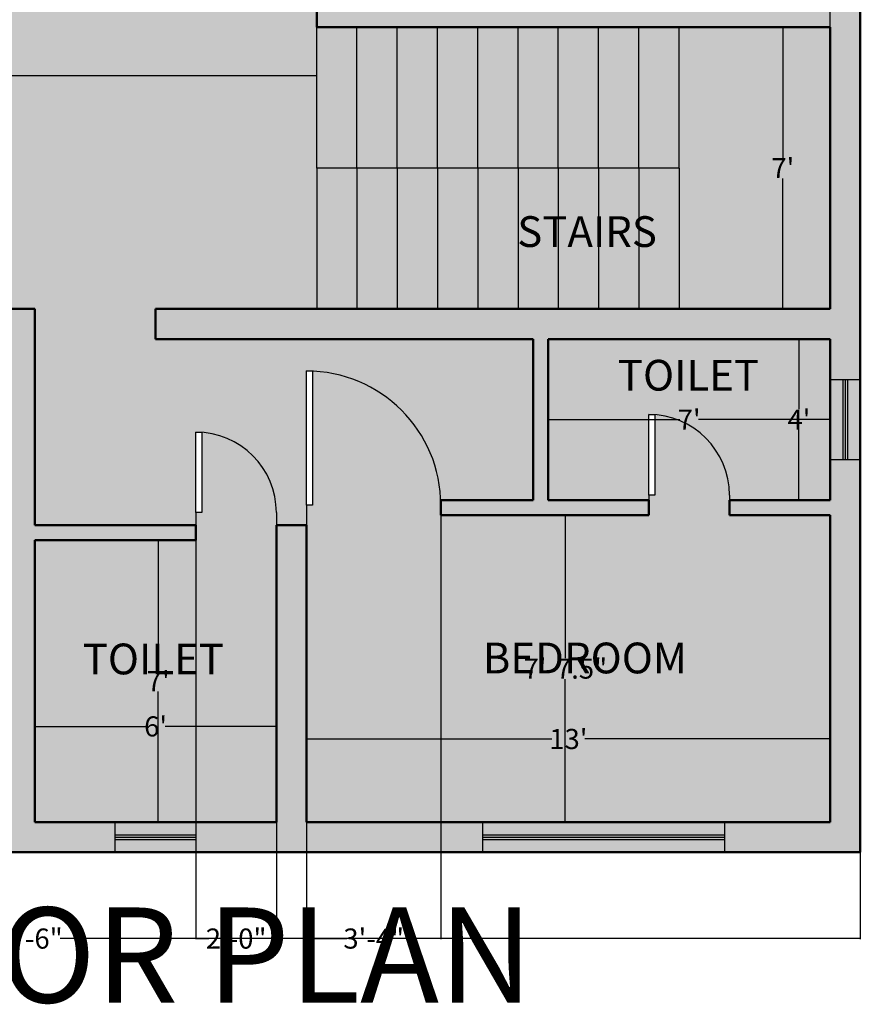
# Model space of a CAD drawing. Units: inches. Extents: x 1379 to 6665, y -118 to 1026.
# Tile 28 of 29: x 6415 to 6665, y 26 to 320. Entities that reach past the tile are written whole.
import ezdxf

# ---------------------------------------------------------------- set-up
doc = ezdxf.new("R2010")
doc.units = ezdxf.units.IN
doc.header["$MEASUREMENT"] = 0
for name, color, linetype, lineweight in [('A-ANNO-DIMS', 2, 'Continuous', 18), ('A-ANNO-TEXT', 7, 'Continuous', 35), ('A-AREA-IDEN', 7, 'Continuous', 25), ('A-DOOR', 1, 'Continuous', 25), ('A-FLOR-PATT', 252, 'Continuous', 13), ('A-FLOR-STRS', 131, 'Continuous', 25), ('A-GLAZ', 2, 'Continuous', 25), ('A-WALL', 7, 'Continuous', 50), ('A-WALL-PATT', 8, 'Continuous', 13)]:
    doc.layers.add(name, color=color, linetype=linetype, lineweight=lineweight)
doc.styles.get("Standard").update_dxf_attribs({"font": 'arial.ttf'})
doc.dimstyles.get("Standard").update_dxf_attribs({"dimtxt": 6, "dimasz": 0.18, "dimexe": 0.18, "dimexo": 0.0625, "dimgap": 0.09, "dimtad": 0, "dimtih": 1, "dimtoh": 1, "dimdec": 1, "dimzin": 0, "dimdsep": 46, "dimlunit": 3, "dimtxsty": 'Standard', "dimcen": 0.09, "dimclrt": 250, "dimadec": 0, "dimazin": 0, "dimtfac": 1, "dimtdec": 1, "dimtofl": 0, "dimtmove": 0, "dimatfit": 3, "dimfxl": 1, "dimtolj": 1, "dimtzin": 0, "dimarcsym": 0})

# ---------------------------------------------------------------- blocks, each defined once
blk = doc.blocks.new('*D79')
at = {"layer": 'A-ANNO-DIMS', "color": 0, "lineweight": -2, "transparency": 16777216}
for p, q in [((6640.02, 317.64), (6642.5, 317.64)), ((6642.32, 317.46), (6642.32, 278.73)), ((6642.32, 233.82), (6642.32, 272.55)), ((6640.02, 233.64), (6642.5, 233.64))]:
    blk.add_line(p, q, dxfattribs=at)
at = {"layer": 'A-ANNO-DIMS', "color": 0, "transparency": 16777216}
for points in [[(6642.29, 317.46), (6642.35, 317.46), (6642.32, 317.64)], [(6642.29, 233.82), (6642.35, 233.82), (6642.32, 233.64)]]:
    blk.add_solid(points, dxfattribs=at)
at = {"layer": 'Defpoints', "color": 0, "transparency": 16777216}
for p in [(6639.95, 317.64), (6639.95, 233.64), (6642.32, 233.64)]:
    blk.add_point(p, dxfattribs=at)
at = {"layer": 'A-ANNO-DIMS', "color": 0, "transparency": 16777216, "insert": (6642.32, 275.64), "char_height": 6, "attachment_point": 5}
blk.add_mtext("\\A1;7'", dxfattribs=at)
blk = doc.blocks.new('*U2')
for p, q in [((0, 0), (0, -6)), ((24, 0), (24, -6))]:
    blk.add_line(p, q)
blk.add_lwpolyline([(0, 0), (0, 24), (1.75, 24), (1.75, 0)], close=True)
blk.add_arc((0, 0), 24, 0, 90)
blk = doc.blocks.new('*U25')
for p, q in [((0, 0), (0, -6)), ((40, 0), (40, -6))]:
    blk.add_line(p, q)
blk.add_lwpolyline([(0, 0), (0, 40), (1.75, 40), (1.75, 0)], close=True)
blk.add_arc((0, 0), 40, 0, 90)
blk = doc.blocks.new('*D80')
at = {"layer": 'A-ANNO-DIMS', "color": 0, "lineweight": -2, "transparency": 16777216}
for p, q in [((6176.4, 282.22), (6176.4, 303.33)), ((6176.58, 303.15), (6325.96, 303.15)), ((6503.22, 303.15), (6353.84, 303.15)), ((6503.4, 282.22), (6503.4, 303.33))]:
    blk.add_line(p, q, dxfattribs=at)
at = {"layer": 'A-ANNO-DIMS', "color": 0, "transparency": 16777216}
for points in [[(6176.58, 303.18), (6176.58, 303.12), (6176.4, 303.15)], [(6503.22, 303.18), (6503.22, 303.12), (6503.4, 303.15)]]:
    blk.add_solid(points, dxfattribs=at)
at = {"layer": 'Defpoints', "color": 0, "transparency": 16777216}
for p in [(6503.4, 303.15), (6176.4, 282.16), (6503.4, 282.16)]:
    blk.add_point(p, dxfattribs=at)
at = {"layer": 'A-ANNO-DIMS', "color": 0, "transparency": 16777216, "insert": (6339.9, 303.15), "char_height": 6, "attachment_point": 5}
blk.add_mtext('\\A1;27\'-3.0"', dxfattribs=at)
blk = doc.blocks.new('*D70')
at = {"layer": 'A-ANNO-DIMS', "color": 0, "lineweight": -2, "transparency": 16777216}
for p, q in [((6453.93, 164.64), (6456.37, 164.64)), ((6456.19, 164.46), (6456.19, 125.73)), ((6456.19, 80.82), (6456.19, 119.55)), ((6453.93, 80.64), (6456.37, 80.64))]:
    blk.add_line(p, q, dxfattribs=at)
at = {"layer": 'A-ANNO-DIMS', "color": 0, "transparency": 16777216}
for points in [[(6456.16, 164.46), (6456.22, 164.46), (6456.19, 164.64)], [(6456.16, 80.82), (6456.22, 80.82), (6456.19, 80.64)]]:
    blk.add_solid(points, dxfattribs=at)
at = {"layer": 'Defpoints', "color": 0, "transparency": 16777216}
for p in [(6453.87, 164.64), (6453.87, 80.64), (6456.19, 80.64)]:
    blk.add_point(p, dxfattribs=at)
at = {"layer": 'A-ANNO-DIMS', "color": 0, "transparency": 16777216, "insert": (6456.19, 122.64), "char_height": 6, "attachment_point": 5}
blk.add_mtext("\\A1;7'", dxfattribs=at)
blk = doc.blocks.new('*D71')
at = {"layer": 'A-ANNO-DIMS', "color": 0, "lineweight": -2, "transparency": 16777216}
for p, q in [((6419.4, 114.02), (6419.4, 108.98)), ((6419.58, 109.16), (6452.54, 109.16)), ((6491.22, 109.16), (6458.27, 109.16)), ((6491.4, 109.22), (6491.4, 109.34))]:
    blk.add_line(p, q, dxfattribs=at)
at = {"layer": 'A-ANNO-DIMS', "color": 0, "transparency": 16777216}
for points in [[(6419.58, 109.19), (6419.58, 109.13), (6419.4, 109.16)], [(6491.22, 109.19), (6491.22, 109.13), (6491.4, 109.16)]]:
    blk.add_solid(points, dxfattribs=at)
at = {"layer": 'Defpoints', "color": 0, "transparency": 16777216}
for p in [(6419.4, 114.09), (6491.4, 109.16), (6491.4, 109.16)]:
    blk.add_point(p, dxfattribs=at)
at = {"layer": 'A-ANNO-DIMS', "color": 0, "transparency": 16777216, "insert": (6455.4, 109.16), "char_height": 6, "attachment_point": 5}
blk.add_mtext("\\A1;6'", dxfattribs=at)
blk = doc.blocks.new('*D72')
at = {"layer": 'A-ANNO-DIMS', "color": 0, "lineweight": -2, "transparency": 16777216}
for p, q in [((6578.31, 172.14), (6577.32, 172.14)), ((6577.5, 171.96), (6577.5, 129.53)), ((6577.5, 80.82), (6577.5, 123.25)), ((6578.31, 80.64), (6577.32, 80.64))]:
    blk.add_line(p, q, dxfattribs=at)
at = {"layer": 'A-ANNO-DIMS', "color": 0, "transparency": 16777216}
for points in [[(6577.47, 171.96), (6577.53, 171.96), (6577.5, 172.14)], [(6577.47, 80.82), (6577.53, 80.82), (6577.5, 80.64)]]:
    blk.add_solid(points, dxfattribs=at)
at = {"layer": 'Defpoints', "color": 0, "transparency": 16777216}
for p in [(6578.37, 172.14), (6577.5, 80.64), (6578.37, 80.64)]:
    blk.add_point(p, dxfattribs=at)
at = {"layer": 'A-ANNO-DIMS', "color": 0, "transparency": 16777216, "insert": (6577.5, 126.39), "char_height": 6, "attachment_point": 5}
blk.add_mtext('\\A1;7\'-7.5"', dxfattribs=at)
blk = doc.blocks.new('*D73')
at = {"layer": 'A-ANNO-DIMS', "color": 0, "lineweight": -2, "transparency": 16777216}
for p, q in [((6500.4, 124.83), (6500.4, 105.22)), ((6656.4, 124.83), (6656.4, 105.22)), ((6500.58, 105.4), (6573.5, 105.4)), ((6656.22, 105.4), (6583.3, 105.4))]:
    blk.add_line(p, q, dxfattribs=at)
at = {"layer": 'A-ANNO-DIMS', "color": 0, "transparency": 16777216}
for points in [[(6500.58, 105.43), (6500.58, 105.37), (6500.4, 105.4)], [(6656.22, 105.43), (6656.22, 105.37), (6656.4, 105.4)]]:
    blk.add_solid(points, dxfattribs=at)
at = {"layer": 'Defpoints', "color": 0, "transparency": 16777216}
for p in [(6500.4, 124.89), (6656.4, 124.89), (6656.4, 105.4)]:
    blk.add_point(p, dxfattribs=at)
at = {"layer": 'A-ANNO-DIMS', "color": 0, "transparency": 16777216, "insert": (6578.4, 105.4), "char_height": 6, "attachment_point": 5}
blk.add_mtext("\\A1;13'", dxfattribs=at)
blk = doc.blocks.new('*D74')
at = {"layer": 'A-ANNO-DIMS', "color": 0, "lineweight": -2, "transparency": 16777216}
for p, q in [((6647.16, 224.64), (6646.93, 224.64)), ((6647.11, 224.46), (6647.11, 203.73)), ((6647.11, 176.82), (6647.11, 197.55)), ((6647.16, 176.64), (6646.93, 176.64))]:
    blk.add_line(p, q, dxfattribs=at)
at = {"layer": 'A-ANNO-DIMS', "color": 0, "transparency": 16777216}
for points in [[(6647.08, 224.46), (6647.14, 224.46), (6647.11, 224.64)], [(6647.08, 176.82), (6647.14, 176.82), (6647.11, 176.64)]]:
    blk.add_solid(points, dxfattribs=at)
at = {"layer": 'Defpoints', "color": 0, "transparency": 16777216}
for p in [(6647.23, 224.64), (6647.11, 176.64), (6647.23, 176.64)]:
    blk.add_point(p, dxfattribs=at)
at = {"layer": 'A-ANNO-DIMS', "color": 0, "transparency": 16777216, "insert": (6647.11, 200.64), "char_height": 6, "attachment_point": 5}
blk.add_mtext("\\A1;4'", dxfattribs=at)
blk = doc.blocks.new('*D75')
at = {"layer": 'A-ANNO-DIMS', "color": 0, "lineweight": -2, "transparency": 16777216}
for p, q in [((6572.4, 194.48), (6572.4, 200.82)), ((6572.58, 200.64), (6611.58, 200.64)), ((6656.22, 200.64), (6617.23, 200.64)), ((6656.4, 191.52), (6656.4, 200.82))]:
    blk.add_line(p, q, dxfattribs=at)
at = {"layer": 'A-ANNO-DIMS', "color": 0, "transparency": 16777216}
for points in [[(6572.58, 200.67), (6572.58, 200.61), (6572.4, 200.64)], [(6656.22, 200.67), (6656.22, 200.61), (6656.4, 200.64)]]:
    blk.add_solid(points, dxfattribs=at)
at = {"layer": 'Defpoints', "color": 0, "transparency": 16777216}
for p in [(6656.4, 200.64), (6572.4, 194.41), (6656.4, 191.46)]:
    blk.add_point(p, dxfattribs=at)
at = {"layer": 'A-ANNO-DIMS', "color": 0, "transparency": 16777216, "insert": (6614.4, 200.64), "char_height": 6, "attachment_point": 5}
blk.add_mtext("\\A1;7'", dxfattribs=at)
blk = doc.blocks.new('WIN-1800')
for p, q in [((0, 0.73), (72, 0.73)), ((0, 0), (72, 0))]:
    blk.add_line(p, q)
blk = doc.blocks.new('WIN-600')
for p, q in [((0, 24), (0, 0)), ((0.73, 24), (0.73, 0))]:
    blk.add_line(p, q)
blk = doc.blocks.new('*D136')
at = {"layer": 'A-ANNO-DIMS', "color": 0, "lineweight": -2, "transparency": 16777216}
for p, q in [((6167.4, 71.58), (6167.4, 45.71)), ((6665.4, 71.58), (6665.4, 45.71)), ((6167.58, 45.89), (6405.89, 45.89)), ((6665.22, 45.89), (6426.92, 45.89))]:
    blk.add_line(p, q, dxfattribs=at)
at = {"layer": 'A-ANNO-DIMS', "color": 0, "transparency": 16777216}
for points in [[(6167.58, 45.92), (6167.58, 45.86), (6167.4, 45.89)], [(6665.22, 45.92), (6665.22, 45.86), (6665.4, 45.89)]]:
    blk.add_solid(points, dxfattribs=at)
at = {"layer": 'Defpoints', "color": 0, "transparency": 16777216}
for p in [(6167.4, 71.64), (6665.4, 71.64), (6665.4, 45.89)]:
    blk.add_point(p, dxfattribs=at)
at = {"layer": 'A-ANNO-DIMS', "color": 250, "transparency": 16777216, "insert": (6416.4, 45.89), "char_height": 6, "attachment_point": 5}
blk.add_mtext('\\A1;41\'-6"', dxfattribs=at)
blk = doc.blocks.new('*D142')
at = {"layer": 'A-ANNO-DIMS', "color": 0, "lineweight": -2, "transparency": 16777216}
for p, q in [((6503.4, 317.7), (6503.4, 529.57)), ((6503.58, 529.39), (6569.79, 529.39)), ((6656.22, 529.39), (6590.02, 529.39)), ((6656.4, 317.7), (6656.4, 529.57))]:
    blk.add_line(p, q, dxfattribs=at)
at = {"layer": 'A-ANNO-DIMS', "color": 0, "transparency": 16777216}
for points in [[(6503.58, 529.42), (6503.58, 529.36), (6503.4, 529.39)], [(6656.22, 529.42), (6656.22, 529.36), (6656.4, 529.39)]]:
    blk.add_solid(points, dxfattribs=at)
at = {"layer": 'Defpoints', "color": 0, "transparency": 16777216}
for p in [(6656.4, 529.39), (6503.4, 317.64), (6656.4, 317.64)]:
    blk.add_point(p, dxfattribs=at)
at = {"layer": 'A-ANNO-DIMS', "color": 250, "transparency": 16777216, "insert": (6579.9, 529.39), "char_height": 6, "attachment_point": 5}
blk.add_mtext('\\A1;12\'-9"', dxfattribs=at)
blk = doc.blocks.new('*D147')
at = {"layer": 'A-ANNO-DIMS', "color": 0, "lineweight": -2, "transparency": 16777216}
for p, q in [((6467.4, 164.58), (6467.4, 45.71)), ((6491.4, 164.58), (6491.4, 45.71)), ((6467.58, 45.89), (6471.29, 45.89)), ((6491.22, 45.89), (6487.52, 45.89))]:
    blk.add_line(p, q, dxfattribs=at)
at = {"layer": 'A-ANNO-DIMS', "color": 0, "transparency": 16777216}
for points in [[(6467.58, 45.92), (6467.58, 45.86), (6467.4, 45.89)], [(6491.22, 45.92), (6491.22, 45.86), (6491.4, 45.89)]]:
    blk.add_solid(points, dxfattribs=at)
at = {"layer": 'Defpoints', "color": 0, "transparency": 16777216}
for p in [(6467.4, 164.64), (6491.4, 164.64), (6491.4, 45.89)]:
    blk.add_point(p, dxfattribs=at)
at = {"layer": 'A-ANNO-DIMS', "color": 250, "transparency": 16777216, "insert": (6479.4, 45.89), "char_height": 6, "attachment_point": 5}
blk.add_mtext('\\A1;2\'-0"', dxfattribs=at)
blk = doc.blocks.new('*D149')
at = {"layer": 'A-ANNO-DIMS', "color": 0, "lineweight": -2, "transparency": 16777216}
for p, q in [((6500.4, 173.33), (6500.4, 45.71)), ((6540.4, 172.08), (6540.4, 45.71)), ((6500.58, 45.89), (6512.34, 45.89)), ((6540.22, 45.89), (6528.46, 45.89))]:
    blk.add_line(p, q, dxfattribs=at)
at = {"layer": 'A-ANNO-DIMS', "color": 0, "transparency": 16777216}
for points in [[(6500.58, 45.92), (6500.58, 45.86), (6500.4, 45.89)], [(6540.22, 45.92), (6540.22, 45.86), (6540.4, 45.89)]]:
    blk.add_solid(points, dxfattribs=at)
at = {"layer": 'Defpoints', "color": 0, "transparency": 16777216}
for p in [(6500.4, 173.39), (6540.4, 172.14), (6540.4, 45.89)]:
    blk.add_point(p, dxfattribs=at)
at = {"layer": 'A-ANNO-DIMS', "color": 250, "transparency": 16777216, "insert": (6520.4, 45.89), "char_height": 6, "attachment_point": 5}
blk.add_mtext('\\A1;3\'-4"', dxfattribs=at)

msp = doc.modelspace()

# ---------------------------------------------------------------- hatches: boundary and pattern name
at = {"layer": 'A-FLOR-PATT', "transparency": 33554590}
h = msp.add_hatch(color=256, dxfattribs=at)
h.dxf.hatch_style = 1
h.paths.add_polyline_path([(6176.4, 382.14), (6176.4, 494.64), (6255.9, 494.64), (6255.9, 503.64), (6167.4, 503.64), (6167.4, 391.14), (6167.4, 323.64), (6176.4, 323.64), (6176.4, 341.64), (6348.9, 341.64), (6348.9, 350.64), (6176.4, 350.64)])
h.paths.add_polyline_path([(6348.9, 233.64), (6176.4, 233.64), (6176.4, 251.64), (6167.4, 251.64), (6167.4, 71.64), (6246.02, 71.64), (6246.02, 80.64), (6176.4, 80.64), (6176.4, 224.64), (6348.9, 224.64)])
h.paths.add_polyline_path([(6443.4, 80.64), (6419.4, 80.64), (6419.4, 164.64), (6467.4, 164.64), (6467.4, 169.14), (6419.4, 169.14), (6419.4, 224.64), (6419.4, 233.64), (6384.87, 233.64), (6384.9, 224.64), (6414.9, 224.64), (6414.9, 80.64), (6318.02, 80.64), (6318.02, 71.64), (6443.4, 71.64)])
h.paths.add_polyline_path([(6552.9, 80.64), (6500.4, 80.64), (6500.4, 169.14), (6491.4, 169.14), (6491.4, 164.64), (6491.4, 80.64), (6467.4, 80.64), (6467.4, 71.64), (6503.4, 71.64), (6552.9, 71.64)])
h.paths.add_polyline_path([(6665.4, 188.64), (6656.4, 188.64), (6656.4, 176.64), (6626.4, 176.64), (6626.4, 172.14), (6656.4, 172.14), (6656.4, 80.64), (6624.9, 80.64), (6624.9, 71.64), (6665.4, 71.64)])
h.paths.add_polyline_path([(6665.4, 503.64), (6614.4, 503.64), (6614.4, 494.64), (6656.4, 494.64), (6656.4, 374.64), (6608.4, 374.64), (6608.4, 370.14), (6656.4, 370.14), (6656.4, 331.14), (6512.4, 331.14), (6503.4, 331.14), (6503.4, 322.14), (6503.4, 317.64), (6656.4, 317.64), (6656.4, 233.64), (6503.4, 233.64), (6455.4, 233.64), (6455.4, 224.64), (6503.4, 224.64), (6567.9, 224.64), (6567.9, 176.64), (6540.4, 176.64), (6540.4, 172.14), (6567.9, 172.14), (6602.4, 172.14), (6602.4, 176.64), (6572.4, 176.64), (6572.4, 224.64), (6656.4, 224.64), (6656.4, 212.64), (6665.4, 212.64)])
h.paths.add_polyline_path([(6584.4, 374.64), (6536.4, 374.64), (6536.4, 370.14), (6536.4, 331.14), (6540.9, 331.14), (6540.9, 370.14), (6584.4, 370.14)], flags=17)
h.paths.add_polyline_path([(6500.4, 494.64), (6542.4, 494.64), (6542.4, 503.64), (6467.4, 503.64), (6467.4, 494.64), (6491.4, 494.64), (6491.4, 370.14), (6500.4, 370.14), (6500.4, 374.64)], flags=17)
h.paths.add_polyline_path([(6443.4, 503.64), (6407.4, 503.64), (6327.9, 503.64), (6327.9, 494.64), (6407.4, 494.64), (6414.9, 494.64), (6414.9, 350.64), (6384.78, 350.64), (6384.9, 341.64), (6419.4, 341.64), (6419.4, 406.14), (6467.4, 406.14), (6467.4, 410.64), (6419.4, 410.64), (6419.4, 494.64), (6443.4, 494.64)])
at = {"layer": 'A-WALL-PATT', "transparency": 33554590}
h = msp.add_hatch(color=256, dxfattribs=at)
h.dxf.hatch_style = 1
h.paths.add_polyline_path([(6414.9, 494.64), (6176.4, 494.64), (6176.4, 382.14), (6176.4, 350.64), (6348.9, 350.64), (6348.9, 383.64), (6350.65, 383.64), (6350.65, 383.6, -0.376042), (6384.78, 350.64), (6414.9, 350.64)])
h.paths.add_polyline_path([(6503.4, 317.64), (6503.4, 322.14), (6503.4, 331.14), (6512.4, 331.14), (6536.4, 331.14), (6536.4, 370.14), (6536.4, 376.14, 0.400041), (6502.15, 412.1), (6502.15, 376.14), (6500.4, 376.14), (6500.4, 370.14), (6491.4, 370.14), (6491.4, 414.39, 0.392996), (6469.15, 438.33), (6469.15, 414.39), (6467.4, 414.39), (6467.4, 408.39), (6467.4, 406.14), (6419.4, 406.14), (6419.4, 341.64), (6384.9, 341.64), (6384.78, 350.64, 0.376042), (6350.65, 383.6), (6350.65, 347.64), (6348.9, 347.64), (6348.9, 341.64), (6176.4, 341.64), (6176.4, 233.64), (6348.9, 233.64), (6348.9, 266.64), (6350.65, 266.64), (6350.65, 266.6, -0.376042), (6384.78, 233.64), (6419.4, 233.64), (6419.4, 224.64), (6419.4, 169.14), (6467.4, 169.14), (6467.4, 172.89), (6467.4, 196.89), (6469.15, 196.89), (6469.15, 196.83, -0.392996), (6491.4, 172.89), (6491.4, 169.14), (6500.4, 169.14), (6500.4, 175.14), (6500.4, 215.14), (6502.15, 215.14), (6502.15, 215.1, -0.390605), (6540.37, 176.64), (6567.9, 176.64), (6567.9, 224.64), (6500.4, 224.64), (6455.4, 224.64), (6455.4, 233.64), (6503.4, 233.64), (6503.4, 275.64)])
h.paths.add_polyline_path([(6491.4, 494.64), (6419.4, 494.64), (6419.4, 410.64), (6467.4, 410.64), (6467.4, 414.39), (6467.4, 438.39), (6469.15, 438.39), (6469.15, 438.33, -0.392996), (6491.4, 414.39)])
h.paths.add_polyline_path([(6656.4, 494.64), (6500.4, 494.64), (6500.4, 412.14), (6502.15, 412.14), (6502.15, 412.1, -0.400041), (6536.4, 376.14), (6536.4, 374.64), (6584.4, 374.64), (6584.4, 376.14), (6584.4, 400.14), (6586.15, 400.14), (6586.15, 400.08, -0.392996), (6608.4, 376.14), (6608.4, 374.64), (6656.4, 374.64)])
h.paths.add_polyline_path([(6414.9, 224.64), (6384.9, 224.64), (6384.87, 233.64), (6384.78, 233.64, 0.376042), (6350.65, 266.6), (6350.65, 266.64), (6348.9, 266.64), (6348.9, 233.64), (6348.9, 224.64), (6176.4, 224.64), (6176.4, 80.64), (6414.9, 80.64)])
h.paths.add_polyline_path([(6491.4, 164.64), (6491.4, 169.14), (6491.4, 172.89, 0.392996), (6469.15, 196.83), (6469.15, 172.89), (6467.4, 172.89), (6467.4, 169.14), (6467.4, 166.89), (6467.4, 164.64), (6419.4, 164.64), (6419.4, 80.64), (6491.4, 80.64)])
h.paths.add_polyline_path([(6656.4, 172.14), (6626.4, 172.14), (6626.4, 178.14, 0.392996), (6604.15, 202.08), (6604.15, 178.14), (6602.4, 178.14), (6602.4, 172.14), (6567.9, 172.14), (6540.4, 172.14), (6540.4, 175.14, 0.401453), (6502.15, 215.1), (6502.15, 175.14), (6500.4, 175.14), (6500.4, 169.14), (6500.4, 80.64), (6503.4, 80.64), (6656.4, 80.64)])
h.paths.add_polyline_path([(6656.4, 224.64), (6572.4, 224.64), (6572.4, 176.64), (6602.4, 176.64), (6602.4, 178.14), (6602.4, 202.14), (6604.15, 202.14), (6604.15, 202.08, -0.392996), (6626.4, 178.14), (6626.4, 176.64), (6656.4, 176.64)])
h.paths.add_polyline_path([(6656.4, 370.14), (6608.4, 370.14), (6608.4, 376.14, 0.392996), (6586.15, 400.08), (6586.15, 376.14), (6584.4, 376.14), (6584.4, 374.64), (6584.4, 370.14), (6540.9, 370.14), (6540.9, 331.14), (6656.4, 331.14)])
h.paths.add_polyline_path([(6259.03, 431.04), (6329.97, 431.04), (6329.97, 445.28), (6259.03, 445.28)], flags=24)
h.paths.add_polyline_path([(6256.77, 281.02), (6365.45, 281.02), (6365.45, 295.25), (6256.77, 295.25)], flags=24)
h.paths.add_polyline_path([(6437.04, 454.45), (6486.63, 454.45), (6486.63, 468.69), (6437.04, 468.69)], flags=24)
h.paths.add_polyline_path([(6549.24, 450.74), (6620.18, 450.74), (6620.18, 464.98), (6549.24, 464.98)], flags=24)
h.paths.add_polyline_path([(6259.03, 146.52), (6329.97, 146.52), (6329.97, 160.75), (6259.03, 160.75)], flags=24)
h.paths.add_polyline_path([(6431.31, 122.15), (6480.89, 122.15), (6480.89, 136.39), (6431.31, 136.39)], flags=24)
h.paths.add_polyline_path([(6550.53, 122.44), (6621.47, 122.44), (6621.47, 136.68), (6550.53, 136.68)], flags=24)
h.paths.add_polyline_path([(6590.78, 206.76), (6640.36, 206.76), (6640.36, 221), (6590.78, 221)], flags=24)
h.paths.add_polyline_path([(6574.95, 341.57), (6624.53, 341.57), (6624.53, 355.8), (6574.95, 355.8)], flags=24)
h = msp.add_hatch(color=256, dxfattribs=at)
h.dxf.hatch_style = 1
h.paths.add_polyline_path([(6575.4, 317.64), (6563.4, 317.64), (6563.4, 275.64), (6575.4, 275.64)])
h.paths.add_polyline_path([(6563.4, 317.64), (6551.4, 317.64), (6551.4, 275.64), (6563.4, 275.64)])
h.paths.add_polyline_path([(6551.4, 317.64), (6539.4, 317.64), (6539.4, 275.64), (6551.4, 275.64)])
h.paths.add_polyline_path([(6539.4, 317.64), (6527.4, 317.64), (6527.4, 275.64), (6539.4, 275.64)])
h.paths.add_polyline_path([(6527.4, 317.64), (6515.4, 317.64), (6515.4, 275.64), (6527.4, 275.64)])
h.paths.add_polyline_path([(6515.4, 317.64), (6503.4, 317.64), (6503.4, 275.64), (6515.4, 275.64)])
h.paths.add_polyline_path([(6587.4, 317.64), (6575.4, 317.64), (6575.4, 275.64), (6587.4, 275.64)])
h.paths.add_polyline_path([(6599.4, 317.64), (6587.4, 317.64), (6587.4, 275.64), (6599.4, 275.64)])
h.paths.add_polyline_path([(6611.4, 317.64), (6599.4, 317.64), (6599.4, 275.64), (6611.4, 275.64)])
h.paths.add_polyline_path([(6611.4, 275.64), (6599.4, 275.64), (6599.4, 233.64), (6611.4, 233.64)])
h.paths.add_polyline_path([(6587.4, 275.64), (6575.4, 275.64), (6575.4, 233.64), (6587.4, 233.64)])
h.paths.add_polyline_path([(6575.4, 275.64), (6563.4, 275.64), (6563.4, 233.64), (6575.4, 233.64)])
h.paths.add_polyline_path([(6563.4, 275.64), (6551.4, 275.64), (6551.4, 233.64), (6563.4, 233.64)])
h.paths.add_polyline_path([(6539.4, 275.64), (6527.4, 275.64), (6527.4, 233.64), (6539.4, 233.64)])
h.paths.add_polyline_path([(6551.4, 275.64), (6539.4, 275.64), (6539.4, 233.64), (6551.4, 233.64)])
h.paths.add_polyline_path([(6527.4, 275.64), (6515.4, 275.64), (6515.4, 233.64), (6527.4, 233.64)])
h.paths.add_polyline_path([(6515.4, 275.64), (6503.4, 275.64), (6503.4, 233.64), (6515.4, 233.64)])
h.paths.add_polyline_path([(6599.4, 275.64), (6587.4, 275.64), (6587.4, 233.64), (6599.4, 233.64)])
h.paths.add_polyline_path([(6656.4, 317.64), (6611.4, 317.64), (6611.4, 275.64), (6611.4, 233.64), (6656.4, 233.64)])
h.paths.add_polyline_path([(6560.8, 249.6), (6611.81, 249.6), (6611.81, 263.82), (6560.8, 263.82)], flags=9)
h = msp.add_hatch(color=256, dxfattribs=at)
h.dxf.hatch_style = 1
h.paths.add_polyline_path([(6665.4, 188.64), (6665.4, 212.64), (6661.63, 212.64), (6661.63, 188.64)])
h.paths.add_polyline_path([(6660.17, 188.64), (6660.17, 212.64), (6656.4, 212.64), (6656.4, 188.64)])
h.paths.add_polyline_path([(6660.9, 188.64), (6660.9, 212.64), (6660.17, 212.64), (6660.17, 188.64)])
h.paths.add_polyline_path([(6661.63, 188.64), (6661.63, 212.64), (6660.9, 212.64), (6660.9, 188.64)])
h = msp.add_hatch(color=256, dxfattribs=at)
h.dxf.hatch_style = 1
h.paths.add_polyline_path([(6467.4, 80.64), (6443.4, 80.64), (6443.4, 76.87), (6467.4, 76.87)])
h.paths.add_polyline_path([(6467.4, 75.41), (6443.4, 75.41), (6443.4, 71.64), (6467.4, 71.64)])
h.paths.add_polyline_path([(6467.4, 76.14), (6443.4, 76.14), (6443.4, 75.41), (6467.4, 75.41)])
h.paths.add_polyline_path([(6467.4, 76.87), (6443.4, 76.87), (6443.4, 76.14), (6467.4, 76.14)])
at = {"layer": 'A-WALL-PATT', "transparency": 33554564}
h = msp.add_hatch(color=256, dxfattribs=at)
h.dxf.hatch_style = 1
h.paths.add_polyline_path([(6624.9, 80.64), (6552.9, 80.64), (6552.9, 76.87), (6624.9, 76.87)])
h.paths.add_polyline_path([(6624.9, 76.14), (6552.9, 76.14), (6552.9, 75.41), (6624.9, 75.41)])
h.paths.add_polyline_path([(6624.9, 76.87), (6552.9, 76.87), (6552.9, 76.14), (6624.9, 76.14)])
h.paths.add_polyline_path([(6624.9, 75.41), (6552.9, 75.41), (6552.9, 71.64), (6624.9, 71.64)])

# ---------------------------------------------------------------- linework, layer by layer
at = {"layer": 'A-FLOR-STRS'}
for p, q in [((6503.4, 275.64), (6503.4, 317.64)), ((6515.4, 275.64), (6515.4, 317.64)), ((6527.4, 275.64), (6527.4, 317.64)), ((6539.4, 275.64), (6539.4, 317.64)), ((6551.4, 275.64), (6551.4, 317.64)), ((6563.4, 275.64), (6563.4, 317.64)), ((6575.4, 275.64), (6575.4, 317.64)), ((6587.4, 275.64), (6587.4, 317.64)), ((6599.4, 275.64), (6599.4, 317.64)), ((6611.4, 275.64), (6611.4, 317.64)), ((6611.4, 275.64), (6503.4, 275.64)), ((6503.4, 275.64), (6503.4, 233.64)), ((6515.4, 275.64), (6515.4, 233.64)), ((6527.4, 275.64), (6527.4, 233.64)), ((6539.4, 275.64), (6539.4, 233.64)), ((6551.4, 275.64), (6551.4, 233.64)), ((6563.4, 275.64), (6563.4, 233.64)), ((6575.4, 275.64), (6575.4, 233.64)), ((6587.4, 275.64), (6587.4, 233.64)), ((6599.4, 275.64), (6599.4, 233.64)), ((6611.4, 275.64), (6611.4, 233.64))]:
    msp.add_line(p, q, dxfattribs=at)
at = {"layer": 'A-GLAZ'}
for p, q in [((6660.17, 212.64), (6660.17, 188.64)), ((6443.4, 75.41), (6467.4, 75.41)), ((6552.9, 75.41), (6624.9, 75.41))]:
    msp.add_line(p, q, dxfattribs=at)
for points in [[(6665.4, 212.64), (6665.4, 188.64), (6656.4, 188.64), (6656.4, 212.64)], [(6443.4, 80.64), (6467.4, 80.64), (6467.4, 71.64), (6443.4, 71.64)], [(6552.9, 80.64), (6624.9, 80.64), (6624.9, 71.64), (6552.9, 71.64)]]:
    msp.add_lwpolyline(points, close=True, dxfattribs=at)
at = {"layer": 'A-WALL'}
for p, q in [((6665.4, 503.64), (6665.4, 71.64)), ((6503.4, 322.14), (6503.4, 317.64)), ((6656.4, 317.64), (6503.4, 317.64)), ((6656.4, 317.64), (6656.4, 233.64)), ((6419.4, 233.64), (6384.87, 233.64)), ((6419.4, 224.64), (6419.4, 233.64)), ((6503.4, 233.64), (6455.4, 233.64)), ((6455.4, 224.64), (6455.4, 233.64)), ((6656.4, 233.64), (6503.4, 233.64)), ((6419.4, 224.64), (6419.4, 169.14)), ((6503.4, 224.64), (6455.4, 224.64)), ((6567.9, 224.64), (6500.4, 224.64)), ((6567.9, 224.64), (6567.9, 176.64)), ((6572.4, 224.64), (6572.4, 176.64)), ((6656.4, 224.64), (6572.4, 224.64)), ((6656.4, 224.64), (6656.4, 176.64)), ((6567.9, 176.64), (6540.4, 176.64)), ((6540.4, 176.64), (6540.4, 172.14)), ((6602.4, 176.64), (6572.4, 176.64)), ((6602.4, 176.64), (6602.4, 172.14)), ((6656.4, 176.64), (6626.4, 176.64)), ((6626.4, 176.64), (6626.4, 172.14)), ((6567.9, 172.14), (6540.4, 172.14)), ((6602.4, 172.14), (6567.9, 172.14)), ((6656.4, 172.14), (6626.4, 172.14)), ((6656.4, 172.14), (6656.4, 80.64)), ((6467.4, 169.14), (6419.4, 169.14)), ((6467.4, 164.64), (6467.4, 169.14)), ((6500.4, 169.14), (6491.4, 169.14)), ((6491.4, 164.64), (6491.4, 169.14)), ((6500.4, 169.14), (6500.4, 80.64)), ((6419.4, 164.64), (6419.4, 80.64)), ((6467.4, 164.64), (6419.4, 164.64)), ((6491.4, 164.64), (6491.4, 80.64)), ((6491.4, 80.64), (6419.4, 80.64)), ((6656.4, 80.64), (6500.4, 80.64)), ((6503.4, 80.64), (6500.4, 80.64)), ((6503.4, 71.64), (6167.4, 71.64)), ((6665.4, 71.64), (6503.4, 71.64))]:
    msp.add_line(p, q, dxfattribs=at)

# ---------------------------------------------------------------- block references
at = {"layer": 'A-DOOR'}
for name, p in [('*U25', (6500.4, 175.14)), ('*U2', (6602.4, 178.14)), ('*U2', (6467.4, 172.89))]:
    msp.add_blockref(name, p, dxfattribs=at)
at = {"layer": 'A-GLAZ'}
for name, p in [('WIN-600', (6660.9, 188.64)), ('WIN-1800', (6552.9, 76.14))]:
    msp.add_blockref(name, p, dxfattribs=at)
at = {"layer": 'A-GLAZ', "rotation": 90.00000000000153}
msp.add_blockref('WIN-600', (6467.4, 76.14), dxfattribs=at)

# ---------------------------------------------------------------- texts
at = {"layer": 'A-ANNO-TEXT'}
msp.add_text('FIRST FLOOR PLAN', height=28.3655, dxfattribs=at).set_placement((6225.6, 26.79))
at = {"layer": 'A-AREA-IDEN'}
for s, p in [('STAIRS', (6563.17, 252.12)), ('TOILET', (6593.15, 209.29)), ('TOILET', (6433.68, 124.68)), ('BEDROOM', (6552.9, 124.97))]:
    msp.add_text(s, height=9.17, dxfattribs=at).set_placement(p)

# ---------------------------------------------------------------- dimensions: what is measured, and where the dimension line sits
at = {"layer": 'A-ANNO-DIMS'}
for base, p1, p2, override, picture, middle in [((6656.4, 529.39), (6503.4, 317.64), (6656.4, 317.64), {"dimdec": 1, "dimlfac": 1, "dimrnd": 0, "dimzin": 1, "dimdsep": 46, "dimlunit": 4, "dimfrac": 2}, '*D142', (6579.9, 529.39)), ((6503.4, 303.15), (6176.4, 282.16), (6503.4, 282.16), {"dimclrd": 0, "dimclre": 0, "dimclrt": 0}, '*D80', (6339.9, 303.15)), ((6656.4, 200.64), (6572.4, 194.41), (6656.4, 191.46), {"dimclrd": 0, "dimclre": 0, "dimclrt": 0}, '*D75', (6614.4, 200.64)), ((6540.4, 45.89), (6500.4, 173.39), (6540.4, 172.14), {"dimdec": 1, "dimlfac": 1, "dimrnd": 0, "dimzin": 1, "dimdsep": 46, "dimlunit": 4, "dimfrac": 2}, '*D149', (6520.4, 45.89)), ((6491.4, 45.89), (6467.4, 164.64), (6491.4, 164.64), {"dimdec": 1, "dimlfac": 1, "dimrnd": 0, "dimzin": 1, "dimdsep": 46, "dimlunit": 4, "dimfrac": 2}, '*D147', (6479.4, 45.89)), ((6656.4, 105.4), (6500.4, 124.89), (6656.4, 124.89), {"dimclrd": 0, "dimclre": 0, "dimclrt": 0}, '*D73', (6578.4, 105.4)), ((6491.4, 109.16), (6419.4, 114.09), (6491.4, 109.16), {"dimclrd": 0, "dimclre": 0, "dimclrt": 0}, '*D71', (6455.4, 109.16)), ((6665.4, 45.89), (6167.4, 71.64), (6665.4, 71.64), {"dimdec": 1, "dimlfac": 1, "dimrnd": 0, "dimzin": 1, "dimdsep": 46, "dimlunit": 4, "dimfrac": 2}, '*D136', (6416.4, 45.89))]:
    dim = msp.add_linear_dim(base=base, p1=p1, p2=p2, dimstyle='Standard', override=override, dxfattribs=at)
    dim.commit()
    dim.dimension.update_dxf_attribs({"geometry": picture, "text_midpoint": middle})
for base, p1, p2, picture, middle in [((6642.32, 233.64), (6639.95, 317.64), (6639.95, 233.64), '*D79', (6642.32, 275.64)), ((6647.11, 176.64), (6647.23, 224.64), (6647.23, 176.64), '*D74', (6647.11, 200.64)), ((6577.5, 80.64), (6578.37, 172.14), (6578.37, 80.64), '*D72', (6577.5, 126.39)), ((6456.19, 80.64), (6453.87, 164.64), (6453.87, 80.64), '*D70', (6456.19, 122.64))]:
    dim = msp.add_linear_dim(base=base, p1=p1, p2=p2, angle=90, dimstyle='Standard', override={"dimclrd": 0, "dimclre": 0, "dimclrt": 0}, dxfattribs=at)
    dim.commit()
    dim.dimension.update_dxf_attribs({"geometry": picture, "text_midpoint": middle})

doc.saveas('drawing.dxf')
